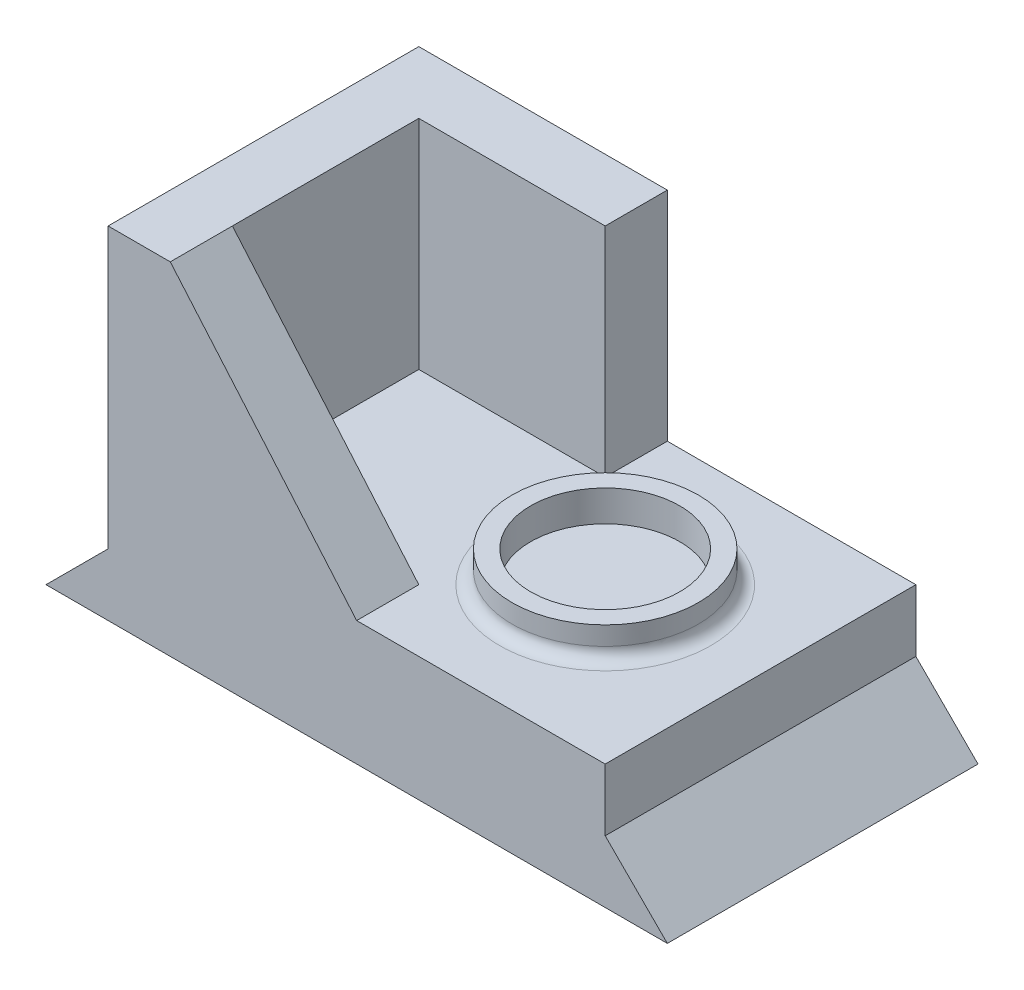
ISO-10303-21;
HEADER;
FILE_DESCRIPTION(('STEP AP214'),'2;1');
FILE_NAME('part.step','',(''),(''),'','','');
FILE_SCHEMA(('AUTOMOTIVE_DESIGN { 1 0 10303 214 1 1 1 1 }'));
ENDSEC;
DATA;
#1=APPLICATION_CONTEXT('core data for automotive mechanical design processes');
#2=APPLICATION_PROTOCOL_DEFINITION('international standard','automotive_design',2000,#1);
#3=PRODUCT_CONTEXT('',#1,'mechanical');
#4=PRODUCT('Part','Part','',(#3));
#5=PRODUCT_RELATED_PRODUCT_CATEGORY('part','',(#4));
#6=PRODUCT_DEFINITION_FORMATION('','',#4);
#7=PRODUCT_DEFINITION_CONTEXT('part definition',#1,'design');
#8=PRODUCT_DEFINITION('design','',#6,#7);
#9=PRODUCT_DEFINITION_SHAPE('','',#8);
#10=(LENGTH_UNIT() NAMED_UNIT(*) SI_UNIT(.MILLI.,.METRE.));
#11=(NAMED_UNIT(*) PLANE_ANGLE_UNIT() SI_UNIT($,.RADIAN.));
#12=(NAMED_UNIT(*) SI_UNIT($,.STERADIAN.) SOLID_ANGLE_UNIT());
#13=UNCERTAINTY_MEASURE_WITH_UNIT(LENGTH_MEASURE(1.E-05),#10,'distance_accuracy_value','');
#14=(GEOMETRIC_REPRESENTATION_CONTEXT(3) GLOBAL_UNCERTAINTY_ASSIGNED_CONTEXT((#13)) GLOBAL_UNIT_ASSIGNED_CONTEXT((#10,
#11,#12)) REPRESENTATION_CONTEXT('',''));
#15=CARTESIAN_POINT('',(0.,0.,0.));
#16=DIRECTION('',(0.,0.,1.));
#17=DIRECTION('',(1.,0.,0.));
#18=AXIS2_PLACEMENT_3D('',#15,#16,#17);
#19=CARTESIAN_POINT('',(-30.,55.,0.));
#20=DIRECTION('',(1.,0.,0.));
#21=DIRECTION('',(0.,0.,-1.));
#22=AXIS2_PLACEMENT_3D('',#19,#20,#21);
#23=PLANE('',#22);
#24=DIRECTION('',(0.,0.,1.));
#25=VECTOR('',#24,1.);
#26=CARTESIAN_POINT('',(-30.,55.,0.));
#27=LINE('',#26,#25);
#28=CARTESIAN_POINT('',(-30.,55.,10.));
#29=VERTEX_POINT('',#28);
#30=CARTESIAN_POINT('',(-30.,55.,40.));
#31=VERTEX_POINT('',#30);
#32=EDGE_CURVE('E150',#29,#31,#27,.T.);
#33=ORIENTED_EDGE('',*,*,#32,.T.);
#34=DIRECTION('',(0.,-1.,0.));
#35=VECTOR('',#34,1.);
#36=CARTESIAN_POINT('',(-30.,55.,40.));
#37=LINE('',#36,#35);
#38=CARTESIAN_POINT('',(-30.,20.,40.));
#39=VERTEX_POINT('',#38);
#40=EDGE_CURVE('E155',#31,#39,#37,.T.);
#41=ORIENTED_EDGE('',*,*,#40,.T.);
#42=DIRECTION('',(0.,0.,1.));
#43=VECTOR('',#42,1.);
#44=CARTESIAN_POINT('',(-30.,20.,0.));
#45=LINE('',#44,#43);
#46=CARTESIAN_POINT('',(-30.,20.,10.));
#47=VERTEX_POINT('',#46);
#48=EDGE_CURVE('E161',#47,#39,#45,.T.);
#49=ORIENTED_EDGE('',*,*,#48,.F.);
#50=DIRECTION('',(0.,-1.,0.));
#51=VECTOR('',#50,1.);
#52=CARTESIAN_POINT('',(-30.,55.,10.));
#53=LINE('',#52,#51);
#54=EDGE_CURVE('E182',#29,#47,#53,.T.);
#55=ORIENTED_EDGE('',*,*,#54,.F.);
#56=EDGE_LOOP('',(#33,#41,#49,#55));
#57=FACE_BOUND('',#56,.T.);
#58=ADVANCED_FACE('F41',(#57),#23,.T.);
#59=CARTESIAN_POINT('',(-40.,10.,50.));
#60=DIRECTION('',(0.707106781186547,-0.707106781186548,0.));
#61=DIRECTION('',(0.707106781186548,0.707106781186547,0.));
#62=AXIS2_PLACEMENT_3D('',#59,#60,#61);
#63=PLANE('',#62);
#64=DIRECTION('',(0.,0.,-1.));
#65=VECTOR('',#64,1.);
#66=CARTESIAN_POINT('',(-40.,10.,50.));
#67=LINE('',#66,#65);
#68=CARTESIAN_POINT('',(-40.,10.,50.));
#69=VERTEX_POINT('',#68);
#70=CARTESIAN_POINT('',(-40.,10.,0.));
#71=VERTEX_POINT('',#70);
#72=EDGE_CURVE('E196',#69,#71,#67,.T.);
#73=ORIENTED_EDGE('',*,*,#72,.T.);
#74=DIRECTION('',(-0.707106781186548,-0.707106781186547,0.));
#75=VECTOR('',#74,1.);
#76=CARTESIAN_POINT('',(-40.,10.,0.));
#77=LINE('',#76,#75);
#78=CARTESIAN_POINT('',(-50.,0.,0.));
#79=VERTEX_POINT('',#78);
#80=EDGE_CURVE('E184',#71,#79,#77,.T.);
#81=ORIENTED_EDGE('',*,*,#80,.T.);
#82=DIRECTION('',(0.,0.,-1.));
#83=VECTOR('',#82,1.);
#84=CARTESIAN_POINT('',(-50.,0.,50.));
#85=LINE('',#84,#83);
#86=CARTESIAN_POINT('',(-50.,0.,50.));
#87=VERTEX_POINT('',#86);
#88=EDGE_CURVE('E222',#87,#79,#85,.T.);
#89=ORIENTED_EDGE('',*,*,#88,.F.);
#90=DIRECTION('',(-0.707106781186548,-0.707106781186547,0.));
#91=VECTOR('',#90,1.);
#92=CARTESIAN_POINT('',(-40.,10.,50.));
#93=LINE('',#92,#91);
#94=EDGE_CURVE('E183',#69,#87,#93,.T.);
#95=ORIENTED_EDGE('',*,*,#94,.F.);
#96=EDGE_LOOP('',(#73,#81,#89,#95));
#97=FACE_BOUND('',#96,.T.);
#98=ADVANCED_FACE('F241',(#97),#63,.F.);
#99=CARTESIAN_POINT('',(-50.,0.,50.));
#100=DIRECTION('',(0.,1.,0.));
#101=DIRECTION('',(-1.,0.,0.));
#102=AXIS2_PLACEMENT_3D('',#99,#100,#101);
#103=PLANE('',#102);
#104=DIRECTION('',(0.,0.,-1.));
#105=VECTOR('',#104,1.);
#106=CARTESIAN_POINT('',(50.,0.,50.));
#107=LINE('',#106,#105);
#108=CARTESIAN_POINT('',(50.,0.,50.));
#109=VERTEX_POINT('',#108);
#110=CARTESIAN_POINT('',(50.,0.,0.));
#111=VERTEX_POINT('',#110);
#112=EDGE_CURVE('E217',#109,#111,#107,.T.);
#113=ORIENTED_EDGE('',*,*,#112,.F.);
#114=DIRECTION('',(1.,0.,0.));
#115=VECTOR('',#114,1.);
#116=CARTESIAN_POINT('',(-50.,0.,50.));
#117=LINE('',#116,#115);
#118=EDGE_CURVE('E190',#87,#109,#117,.T.);
#119=ORIENTED_EDGE('',*,*,#118,.F.);
#120=ORIENTED_EDGE('',*,*,#88,.T.);
#121=DIRECTION('',(1.,0.,0.));
#122=VECTOR('',#121,1.);
#123=CARTESIAN_POINT('',(-50.,0.,0.));
#124=LINE('',#123,#122);
#125=EDGE_CURVE('E203',#79,#111,#124,.T.);
#126=ORIENTED_EDGE('',*,*,#125,.T.);
#127=EDGE_LOOP('',(#113,#119,#120,#126));
#128=FACE_BOUND('',#127,.T.);
#129=ADVANCED_FACE('F253',(#128),#103,.F.);
#130=CARTESIAN_POINT('',(50.,0.,50.));
#131=DIRECTION('',(-0.707106781186547,-0.707106781186548,0.));
#132=DIRECTION('',(0.707106781186548,-0.707106781186547,0.));
#133=AXIS2_PLACEMENT_3D('',#130,#131,#132);
#134=PLANE('',#133);
#135=DIRECTION('',(-0.707106781186548,0.707106781186547,0.));
#136=VECTOR('',#135,1.);
#137=CARTESIAN_POINT('',(50.,0.,0.));
#138=LINE('',#137,#136);
#139=CARTESIAN_POINT('',(40.,10.,0.));
#140=VERTEX_POINT('',#139);
#141=EDGE_CURVE('E201',#111,#140,#138,.T.);
#142=ORIENTED_EDGE('',*,*,#141,.T.);
#143=DIRECTION('',(0.,0.,-1.));
#144=VECTOR('',#143,1.);
#145=CARTESIAN_POINT('',(40.,10.,50.));
#146=LINE('',#145,#144);
#147=CARTESIAN_POINT('',(40.,10.,50.));
#148=VERTEX_POINT('',#147);
#149=EDGE_CURVE('E214',#148,#140,#146,.T.);
#150=ORIENTED_EDGE('',*,*,#149,.F.);
#151=DIRECTION('',(-0.707106781186548,0.707106781186547,0.));
#152=VECTOR('',#151,1.);
#153=CARTESIAN_POINT('',(50.,0.,50.));
#154=LINE('',#153,#152);
#155=EDGE_CURVE('E191',#109,#148,#154,.T.);
#156=ORIENTED_EDGE('',*,*,#155,.F.);
#157=ORIENTED_EDGE('',*,*,#112,.T.);
#158=EDGE_LOOP('',(#142,#150,#156,#157));
#159=FACE_BOUND('',#158,.T.);
#160=ADVANCED_FACE('F273',(#159),#134,.F.);
#161=CARTESIAN_POINT('',(40.,10.,50.));
#162=DIRECTION('',(-1.,0.,0.));
#163=DIRECTION('',(0.,0.,1.));
#164=AXIS2_PLACEMENT_3D('',#161,#162,#163);
#165=PLANE('',#164);
#166=DIRECTION('',(0.,1.,0.));
#167=VECTOR('',#166,1.);
#168=CARTESIAN_POINT('',(40.,10.,0.));
#169=LINE('',#168,#167);
#170=CARTESIAN_POINT('',(40.,20.,0.));
#171=VERTEX_POINT('',#170);
#172=EDGE_CURVE('E202',#140,#171,#169,.T.);
#173=ORIENTED_EDGE('',*,*,#172,.T.);
#174=DIRECTION('',(0.,0.,-1.));
#175=VECTOR('',#174,1.);
#176=CARTESIAN_POINT('',(40.,20.,50.));
#177=LINE('',#176,#175);
#178=CARTESIAN_POINT('',(40.,20.,50.));
#179=VERTEX_POINT('',#178);
#180=EDGE_CURVE('E215',#179,#171,#177,.T.);
#181=ORIENTED_EDGE('',*,*,#180,.F.);
#182=DIRECTION('',(0.,1.,0.));
#183=VECTOR('',#182,1.);
#184=CARTESIAN_POINT('',(40.,10.,50.));
#185=LINE('',#184,#183);
#186=EDGE_CURVE('E194',#148,#179,#185,.T.);
#187=ORIENTED_EDGE('',*,*,#186,.F.);
#188=ORIENTED_EDGE('',*,*,#149,.T.);
#189=EDGE_LOOP('',(#173,#181,#187,#188));
#190=FACE_BOUND('',#189,.T.);
#191=ADVANCED_FACE('F269',(#190),#165,.F.);
#192=CARTESIAN_POINT('',(40.,20.,50.));
#193=DIRECTION('',(0.,-1.,0.));
#194=DIRECTION('',(0.,0.,-1.));
#195=AXIS2_PLACEMENT_3D('',#192,#193,#194);
#196=PLANE('',#195);
#197=CARTESIAN_POINT('',(15.,20.,25.));
#198=DIRECTION('',(0.,-1.,0.));
#199=DIRECTION('',(0.,0.,-1.));
#200=AXIS2_PLACEMENT_3D('',#197,#198,#199);
#201=CIRCLE('',#200,17.);
#202=CARTESIAN_POINT('',(15.,20.,8.));
#203=VERTEX_POINT('',#202);
#204=EDGE_CURVE('E11',#203,#203,#201,.T.);
#205=ORIENTED_EDGE('',*,*,#204,.T.);
#206=EDGE_LOOP('',(#205));
#207=FACE_BOUND('',#206,.T.);
#208=DIRECTION('',(-1.,0.,0.));
#209=VECTOR('',#208,1.);
#210=CARTESIAN_POINT('',(40.,20.,40.));
#211=LINE('',#210,#209);
#212=CARTESIAN_POINT('',(0.,20.,40.));
#213=VERTEX_POINT('',#212);
#214=EDGE_CURVE('E57',#213,#39,#211,.T.);
#215=ORIENTED_EDGE('',*,*,#214,.F.);
#216=DIRECTION('',(0.,0.,-1.));
#217=VECTOR('',#216,1.);
#218=CARTESIAN_POINT('',(0.,20.,50.));
#219=LINE('',#218,#217);
#220=CARTESIAN_POINT('',(0.,20.,50.));
#221=VERTEX_POINT('',#220);
#222=EDGE_CURVE('E58',#213,#221,#219,.F.);
#223=ORIENTED_EDGE('',*,*,#222,.T.);
#224=DIRECTION('',(-1.,0.,0.));
#225=VECTOR('',#224,1.);
#226=CARTESIAN_POINT('',(40.,20.,50.));
#227=LINE('',#226,#225);
#228=EDGE_CURVE('E151',#179,#221,#227,.T.);
#229=ORIENTED_EDGE('',*,*,#228,.F.);
#230=ORIENTED_EDGE('',*,*,#180,.T.);
#231=DIRECTION('',(-1.,0.,0.));
#232=VECTOR('',#231,1.);
#233=CARTESIAN_POINT('',(40.,20.,0.));
#234=LINE('',#233,#232);
#235=CARTESIAN_POINT('',(0.,20.,0.));
#236=VERTEX_POINT('',#235);
#237=EDGE_CURVE('E210',#171,#236,#234,.T.);
#238=ORIENTED_EDGE('',*,*,#237,.T.);
#239=DIRECTION('',(0.,0.,1.));
#240=VECTOR('',#239,1.);
#241=CARTESIAN_POINT('',(0.,20.,0.));
#242=LINE('',#241,#240);
#243=CARTESIAN_POINT('',(0.,20.,10.));
#244=VERTEX_POINT('',#243);
#245=EDGE_CURVE('E146',#236,#244,#242,.T.);
#246=ORIENTED_EDGE('',*,*,#245,.T.);
#247=DIRECTION('',(1.,0.,0.));
#248=VECTOR('',#247,1.);
#249=CARTESIAN_POINT('',(0.,20.,10.));
#250=LINE('',#249,#248);
#251=EDGE_CURVE('E174',#47,#244,#250,.T.);
#252=ORIENTED_EDGE('',*,*,#251,.F.);
#253=ORIENTED_EDGE('',*,*,#48,.T.);
#254=EDGE_LOOP('',(#215,#223,#229,#230,#238,#246,#252,#253));
#255=FACE_BOUND('',#254,.T.);
#256=ADVANCED_FACE('F266',(#207,#255),#196,.F.);
#257=CARTESIAN_POINT('',(-40.,20.,50.));
#258=DIRECTION('',(1.,0.,0.));
#259=DIRECTION('',(0.,0.,-1.));
#260=AXIS2_PLACEMENT_3D('',#257,#258,#259);
#261=PLANE('',#260);
#262=DIRECTION('',(0.,-1.,0.));
#263=VECTOR('',#262,1.);
#264=CARTESIAN_POINT('',(-40.,20.,50.));
#265=LINE('',#264,#263);
#266=CARTESIAN_POINT('',(-40.,55.,50.));
#267=VERTEX_POINT('',#266);
#268=EDGE_CURVE('E198',#267,#69,#265,.T.);
#269=ORIENTED_EDGE('',*,*,#268,.F.);
#270=DIRECTION('',(0.,0.,1.));
#271=VECTOR('',#270,1.);
#272=CARTESIAN_POINT('',(-40.,55.,0.));
#273=LINE('',#272,#271);
#274=CARTESIAN_POINT('',(-40.,55.,0.));
#275=VERTEX_POINT('',#274);
#276=EDGE_CURVE('E131',#275,#267,#273,.T.);
#277=ORIENTED_EDGE('',*,*,#276,.F.);
#278=DIRECTION('',(0.,-1.,0.));
#279=VECTOR('',#278,1.);
#280=CARTESIAN_POINT('',(-40.,20.,0.));
#281=LINE('',#280,#279);
#282=EDGE_CURVE('E186',#275,#71,#281,.T.);
#283=ORIENTED_EDGE('',*,*,#282,.T.);
#284=ORIENTED_EDGE('',*,*,#72,.F.);
#285=EDGE_LOOP('',(#269,#277,#283,#284));
#286=FACE_BOUND('',#285,.T.);
#287=ADVANCED_FACE('F257',(#286),#261,.F.);
#288=CARTESIAN_POINT('',(0.,0.,50.));
#289=DIRECTION('',(0.,0.,-1.));
#290=DIRECTION('',(-1.,0.,0.));
#291=AXIS2_PLACEMENT_3D('',#288,#289,#290);
#292=PLANE('',#291);
#293=ORIENTED_EDGE('',*,*,#228,.T.);
#294=DIRECTION('',(0.650791373455968,-0.759256602365297,0.));
#295=VECTOR('',#294,1.);
#296=CARTESIAN_POINT('',(-30.,55.,50.));
#297=LINE('',#296,#295);
#298=CARTESIAN_POINT('',(-30.,55.,50.));
#299=VERTEX_POINT('',#298);
#300=EDGE_CURVE('E145',#299,#221,#297,.T.);
#301=ORIENTED_EDGE('',*,*,#300,.F.);
#302=DIRECTION('',(1.,0.,0.));
#303=VECTOR('',#302,1.);
#304=CARTESIAN_POINT('',(0.,55.,50.));
#305=LINE('',#304,#303);
#306=EDGE_CURVE('E127',#267,#299,#305,.T.);
#307=ORIENTED_EDGE('',*,*,#306,.F.);
#308=ORIENTED_EDGE('',*,*,#268,.T.);
#309=ORIENTED_EDGE('',*,*,#94,.T.);
#310=ORIENTED_EDGE('',*,*,#118,.T.);
#311=ORIENTED_EDGE('',*,*,#155,.T.);
#312=ORIENTED_EDGE('',*,*,#186,.T.);
#313=EDGE_LOOP('',(#293,#301,#307,#308,#309,#310,#311,#312));
#314=FACE_BOUND('',#313,.T.);
#315=ADVANCED_FACE('F147',(#314),#292,.F.);
#316=CARTESIAN_POINT('',(0.,0.,0.));
#317=DIRECTION('',(0.,0.,-1.));
#318=DIRECTION('',(-1.,0.,0.));
#319=AXIS2_PLACEMENT_3D('',#316,#317,#318);
#320=PLANE('',#319);
#321=ORIENTED_EDGE('',*,*,#80,.F.);
#322=ORIENTED_EDGE('',*,*,#282,.F.);
#323=DIRECTION('',(-1.,0.,0.));
#324=VECTOR('',#323,1.);
#325=CARTESIAN_POINT('',(0.,55.,0.));
#326=LINE('',#325,#324);
#327=CARTESIAN_POINT('',(0.,55.,0.));
#328=VERTEX_POINT('',#327);
#329=EDGE_CURVE('E169',#328,#275,#326,.T.);
#330=ORIENTED_EDGE('',*,*,#329,.F.);
#331=DIRECTION('',(0.,-1.,0.));
#332=VECTOR('',#331,1.);
#333=CARTESIAN_POINT('',(0.,55.,0.));
#334=LINE('',#333,#332);
#335=EDGE_CURVE('E139',#328,#236,#334,.T.);
#336=ORIENTED_EDGE('',*,*,#335,.T.);
#337=ORIENTED_EDGE('',*,*,#237,.F.);
#338=ORIENTED_EDGE('',*,*,#172,.F.);
#339=ORIENTED_EDGE('',*,*,#141,.F.);
#340=ORIENTED_EDGE('',*,*,#125,.F.);
#341=EDGE_LOOP('',(#321,#322,#330,#336,#337,#338,#339,#340));
#342=FACE_BOUND('',#341,.T.);
#343=ADVANCED_FACE('F259',(#342),#320,.T.);
#344=CARTESIAN_POINT('',(0.,55.,10.));
#345=DIRECTION('',(0.,0.,-1.));
#346=DIRECTION('',(-1.,0.,0.));
#347=AXIS2_PLACEMENT_3D('',#344,#345,#346);
#348=PLANE('',#347);
#349=ORIENTED_EDGE('',*,*,#251,.T.);
#350=DIRECTION('',(0.,-1.,0.));
#351=VECTOR('',#350,1.);
#352=CARTESIAN_POINT('',(0.,55.,10.));
#353=LINE('',#352,#351);
#354=CARTESIAN_POINT('',(0.,55.,10.));
#355=VERTEX_POINT('',#354);
#356=EDGE_CURVE('E179',#355,#244,#353,.T.);
#357=ORIENTED_EDGE('',*,*,#356,.F.);
#358=DIRECTION('',(1.,0.,0.));
#359=VECTOR('',#358,1.);
#360=CARTESIAN_POINT('',(0.,55.,10.));
#361=LINE('',#360,#359);
#362=EDGE_CURVE('E162',#29,#355,#361,.T.);
#363=ORIENTED_EDGE('',*,*,#362,.F.);
#364=ORIENTED_EDGE('',*,*,#54,.T.);
#365=EDGE_LOOP('',(#349,#357,#363,#364));
#366=FACE_BOUND('',#365,.T.);
#367=ADVANCED_FACE('F254',(#366),#348,.F.);
#368=CARTESIAN_POINT('',(0.,55.,0.));
#369=DIRECTION('',(1.,0.,0.));
#370=DIRECTION('',(0.,0.,-1.));
#371=AXIS2_PLACEMENT_3D('',#368,#369,#370);
#372=PLANE('',#371);
#373=ORIENTED_EDGE('',*,*,#245,.F.);
#374=ORIENTED_EDGE('',*,*,#335,.F.);
#375=DIRECTION('',(0.,0.,1.));
#376=VECTOR('',#375,1.);
#377=CARTESIAN_POINT('',(0.,55.,0.));
#378=LINE('',#377,#376);
#379=EDGE_CURVE('E164',#328,#355,#378,.T.);
#380=ORIENTED_EDGE('',*,*,#379,.T.);
#381=ORIENTED_EDGE('',*,*,#356,.T.);
#382=EDGE_LOOP('',(#373,#374,#380,#381));
#383=FACE_BOUND('',#382,.T.);
#384=ADVANCED_FACE('F298',(#383),#372,.T.);
#385=CARTESIAN_POINT('',(0.,55.,0.));
#386=DIRECTION('',(0.,1.,0.));
#387=DIRECTION('',(0.,0.,1.));
#388=AXIS2_PLACEMENT_3D('',#385,#386,#387);
#389=PLANE('',#388);
#390=EDGE_CURVE('E128',#31,#299,#27,.T.);
#391=ORIENTED_EDGE('',*,*,#390,.F.);
#392=ORIENTED_EDGE('',*,*,#32,.F.);
#393=ORIENTED_EDGE('',*,*,#362,.T.);
#394=ORIENTED_EDGE('',*,*,#379,.F.);
#395=ORIENTED_EDGE('',*,*,#329,.T.);
#396=ORIENTED_EDGE('',*,*,#276,.T.);
#397=ORIENTED_EDGE('',*,*,#306,.T.);
#398=EDGE_LOOP('',(#391,#392,#393,#394,#395,#396,#397));
#399=FACE_BOUND('',#398,.T.);
#400=ADVANCED_FACE('F126',(#399),#389,.T.);
#401=CARTESIAN_POINT('',(-30.,55.,50.));
#402=DIRECTION('',(-0.759256602365297,-0.650791373455968,0.));
#403=DIRECTION('',(0.650791373455968,-0.759256602365297,0.));
#404=AXIS2_PLACEMENT_3D('',#401,#402,#403);
#405=PLANE('',#404);
#406=ORIENTED_EDGE('',*,*,#222,.F.);
#407=DIRECTION('',(0.650791373455968,-0.759256602365297,0.));
#408=VECTOR('',#407,1.);
#409=CARTESIAN_POINT('',(-30.,55.,40.));
#410=LINE('',#409,#408);
#411=EDGE_CURVE('E148',#31,#213,#410,.T.);
#412=ORIENTED_EDGE('',*,*,#411,.F.);
#413=ORIENTED_EDGE('',*,*,#390,.T.);
#414=ORIENTED_EDGE('',*,*,#300,.T.);
#415=EDGE_LOOP('',(#406,#412,#413,#414));
#416=FACE_BOUND('',#415,.T.);
#417=ADVANCED_FACE('F141',(#416),#405,.F.);
#418=CARTESIAN_POINT('',(0.,27.5,40.));
#419=DIRECTION('',(0.,0.,1.));
#420=DIRECTION('',(1.,0.,0.));
#421=AXIS2_PLACEMENT_3D('',#418,#419,#420);
#422=PLANE('',#421);
#423=ORIENTED_EDGE('',*,*,#411,.T.);
#424=ORIENTED_EDGE('',*,*,#214,.T.);
#425=ORIENTED_EDGE('',*,*,#40,.F.);
#426=EDGE_LOOP('',(#423,#424,#425));
#427=FACE_BOUND('',#426,.T.);
#428=ADVANCED_FACE('F307',(#427),#422,.F.);
#429=CARTESIAN_POINT('',(15.,25.,25.));
#430=DIRECTION('',(0.,-1.,0.));
#431=DIRECTION('',(0.,0.,-1.));
#432=AXIS2_PLACEMENT_3D('',#429,#430,#431);
#433=CYLINDRICAL_SURFACE('',#432,15.);
#434=CARTESIAN_POINT('',(15.,22.,25.));
#435=DIRECTION('',(0.,-1.,0.));
#436=DIRECTION('',(0.,0.,-1.));
#437=AXIS2_PLACEMENT_3D('',#434,#435,#436);
#438=CIRCLE('',#437,15.);
#439=CARTESIAN_POINT('',(15.,22.,10.));
#440=VERTEX_POINT('',#439);
#441=EDGE_CURVE('E47',#440,#440,#438,.F.);
#442=ORIENTED_EDGE('',*,*,#441,.T.);
#443=EDGE_LOOP('',(#442));
#444=FACE_BOUND('',#443,.T.);
#445=CARTESIAN_POINT('',(15.,25.,25.));
#446=DIRECTION('',(0.,1.,0.));
#447=DIRECTION('',(0.,0.,1.));
#448=AXIS2_PLACEMENT_3D('',#445,#446,#447);
#449=CIRCLE('',#448,15.);
#450=CARTESIAN_POINT('',(15.,25.,40.));
#451=VERTEX_POINT('',#450);
#452=EDGE_CURVE('E154',#451,#451,#449,.T.);
#453=ORIENTED_EDGE('',*,*,#452,.F.);
#454=EDGE_LOOP('',(#453));
#455=FACE_BOUND('',#454,.T.);
#456=ADVANCED_FACE('F223',(#444,#455),#433,.T.);
#457=CARTESIAN_POINT('',(15.,25.,25.));
#458=DIRECTION('',(0.,1.,0.));
#459=DIRECTION('',(0.,0.,1.));
#460=AXIS2_PLACEMENT_3D('',#457,#458,#459);
#461=PLANE('',#460);
#462=CARTESIAN_POINT('',(15.,25.,25.));
#463=DIRECTION('',(0.,1.,0.));
#464=DIRECTION('',(0.,0.,1.));
#465=AXIS2_PLACEMENT_3D('',#462,#463,#464);
#466=CIRCLE('',#465,12.);
#467=CARTESIAN_POINT('',(15.,25.,37.));
#468=VERTEX_POINT('',#467);
#469=EDGE_CURVE('E435',#468,#468,#466,.T.);
#470=ORIENTED_EDGE('',*,*,#469,.F.);
#471=EDGE_LOOP('',(#470));
#472=FACE_BOUND('',#471,.T.);
#473=ORIENTED_EDGE('',*,*,#452,.T.);
#474=EDGE_LOOP('',(#473));
#475=FACE_BOUND('',#474,.T.);
#476=ADVANCED_FACE('F228',(#472,#475),#461,.T.);
#477=CARTESIAN_POINT('',(15.,22.,25.));
#478=DIRECTION('',(0.,-1.,0.));
#479=DIRECTION('',(0.,0.,-1.));
#480=AXIS2_PLACEMENT_3D('',#477,#478,#479);
#481=TOROIDAL_SURFACE('',#480,17.,2.);
#482=ORIENTED_EDGE('',*,*,#204,.F.);
#483=EDGE_LOOP('',(#482));
#484=FACE_BOUND('',#483,.T.);
#485=ORIENTED_EDGE('',*,*,#441,.F.);
#486=EDGE_LOOP('',(#485));
#487=FACE_BOUND('',#486,.T.);
#488=ADVANCED_FACE('F43',(#484,#487),#481,.F.);
#489=CARTESIAN_POINT('',(15.,20.,25.));
#490=DIRECTION('',(0.,1.,0.));
#491=DIRECTION('',(0.,0.,1.));
#492=AXIS2_PLACEMENT_3D('',#489,#490,#491);
#493=CYLINDRICAL_SURFACE('',#492,12.);
#494=CARTESIAN_POINT('',(15.,20.,25.));
#495=DIRECTION('',(0.,1.,0.));
#496=DIRECTION('',(0.,0.,1.));
#497=AXIS2_PLACEMENT_3D('',#494,#495,#496);
#498=CIRCLE('',#497,12.);
#499=CARTESIAN_POINT('',(15.,20.,37.));
#500=VERTEX_POINT('',#499);
#501=EDGE_CURVE('E431',#500,#500,#498,.T.);
#502=ORIENTED_EDGE('',*,*,#501,.F.);
#503=EDGE_LOOP('',(#502));
#504=FACE_BOUND('',#503,.T.);
#505=ORIENTED_EDGE('',*,*,#469,.T.);
#506=EDGE_LOOP('',(#505));
#507=FACE_BOUND('',#506,.T.);
#508=ADVANCED_FACE('F226',(#504,#507),#493,.F.);
#509=CARTESIAN_POINT('',(15.,20.,25.));
#510=DIRECTION('',(0.,1.,0.));
#511=DIRECTION('',(0.,0.,1.));
#512=AXIS2_PLACEMENT_3D('',#509,#510,#511);
#513=PLANE('',#512);
#514=ORIENTED_EDGE('',*,*,#501,.T.);
#515=EDGE_LOOP('',(#514));
#516=FACE_BOUND('',#515,.T.);
#517=ADVANCED_FACE('F240',(#516),#513,.T.);
#518=CLOSED_SHELL('',(#58,#98,#129,#160,#191,#256,#287,#315,#343,#367,#384,#400,#417,#428,#456,
#476,#488,#508,#517));
#519=MANIFOLD_SOLID_BREP('B2',#518);
#520=ADVANCED_BREP_SHAPE_REPRESENTATION('',(#18,#519),#14);
#521=SHAPE_DEFINITION_REPRESENTATION(#9,#520);
ENDSEC;
END-ISO-10303-21;
